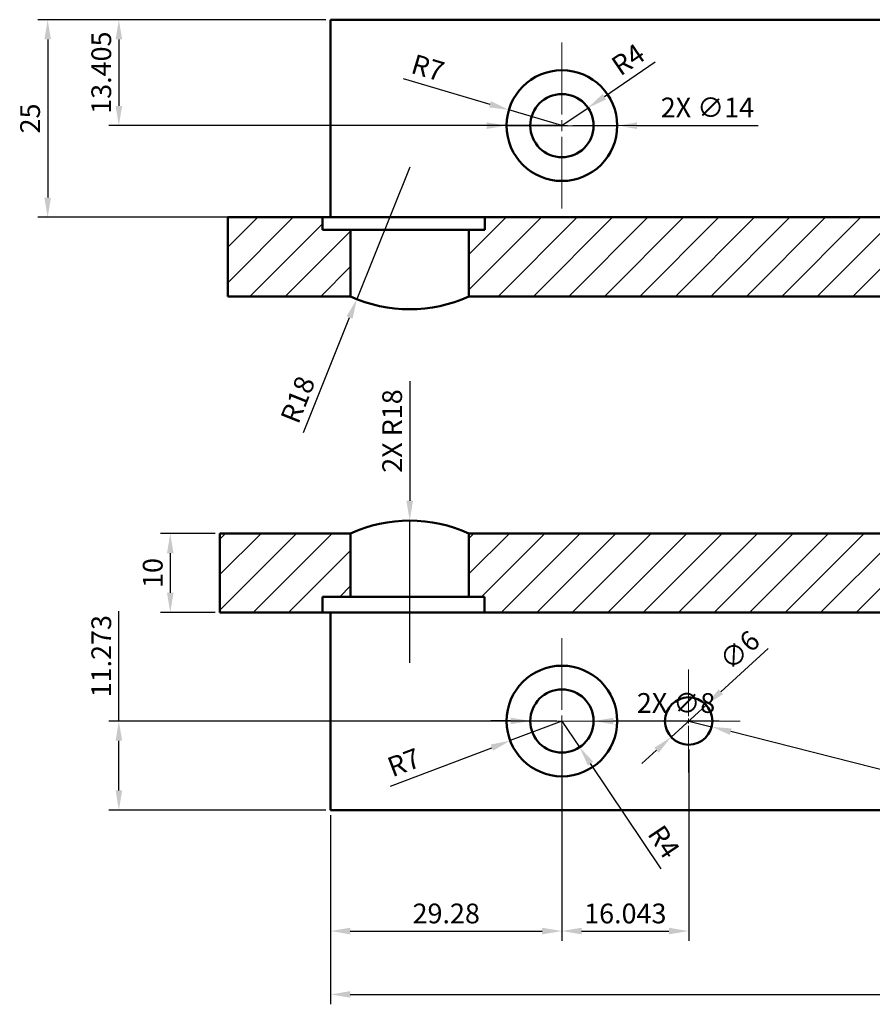
# Model space of a CAD drawing. Units: millimetres. Extents: x 1381 to 2009, y 1325 to 1613.
# Tile 1 of 6: x 1381 to 1489, y 1325 to 1450. Entities that reach past the tile are written whole.
import ezdxf

# ---------------------------------------------------------------- set-up
doc = ezdxf.new("R2010")
doc.units = ezdxf.units.MM
doc.linetypes.add('CENTER', pattern=[50.8, 31.75, -6.35, 6.35, -6.35])
for name, color, linetype, lineweight in [('M-CNTR', 1, 'CENTER', 18), ('M-DIMS', 2, 'Continuous', 25), ('M-HATC', 8, 'Continuous', 18), ('M-OUTL', 7, 'Continuous', 50)]:
    doc.layers.add(name, color=color, linetype=linetype, lineweight=lineweight)
doc.styles.get("Standard").update_dxf_attribs({"font": 'arial.ttf'})
doc.dimstyles.new('ISO-25', dxfattribs={"dimtxt": 2.5, "dimasz": 2.5, "dimexe": 1.25, "dimexo": 0.625, "dimtad": 1, "dimtxsty": 'Standard', "dimcen": 2.5, "dimadec": 0, "dimazin": 0, "dimtfac": 1, "dimtmove": 0, "dimatfit": 3, "dimfxl": 1, "dimarcsym": 0})

# ---------------------------------------------------------------- blocks, each defined once
blk = doc.blocks.new('*U3')
at = {"layer": 'M-CNTR', "color": 0, "transparency": 16777216}
for p, q in [((0, 1.4), (0, 10.5)), ((-10.5, 0), (-1.4, 0)), ((1.4, 0), (10.5, 0)), ((0, -10.5), (0, -1.4))]:
    blk.add_line(p, q, dxfattribs=at)
at = {"layer": 'M-CNTR', "color": 0, "linetype": 'Continuous', "transparency": 16777216}
for p, q in [((-0.7, 0), (0.7, 0)), ((0, -0.7), (0, 0.7))]:
    blk.add_line(p, q, dxfattribs=at)
blk = doc.blocks.new('*U4')
at = {"layer": 'M-CNTR', "color": 0, "transparency": 16777216}
for p, q in [((0, 1.4), (0, 10.5)), ((-10.5, 0), (-1.4, 0)), ((1.4, 0), (10.5, 0)), ((0, -10.5), (0, -1.4))]:
    blk.add_line(p, q, dxfattribs=at)
at = {"layer": 'M-CNTR', "color": 0, "linetype": 'Continuous', "transparency": 16777216}
for p, q in [((-0.7, 0), (0.7, 0)), ((0, -0.7), (0, 0.7))]:
    blk.add_line(p, q, dxfattribs=at)
blk = doc.blocks.new('*U5')
at = {"layer": 'M-CNTR', "color": 0, "transparency": 16777216}
for p, q in [((0, 0.6), (0, 6.5)), ((-6.5, 0), (-0.6, 0)), ((0.6, 0), (6.5, 0)), ((0, -6.5), (0, -0.6))]:
    blk.add_line(p, q, dxfattribs=at)
at = {"layer": 'M-CNTR', "color": 0, "linetype": 'Continuous', "transparency": 16777216}
for p, q in [((-0.3, 0), (0.3, 0)), ((0, -0.3), (0, 0.3))]:
    blk.add_line(p, q, dxfattribs=at)
blk = doc.blocks.new('*D38')
at = {"layer": 'Defpoints', "color": 0, "transparency": 16777216}
for p in [(1420.47, 1349.73), (1600.47, 1349.73), (1600.47, 1326.41)]:
    blk.add_point(p, dxfattribs=at)
at = {"layer": 'M-DIMS', "color": 0, "lineweight": -2, "transparency": 16777216}
for p, q in [((1420.47, 1349.11), (1420.47, 1325.16)), ((1600.47, 1349.11), (1600.47, 1325.16)), ((1422.97, 1326.41), (1597.97, 1326.41))]:
    blk.add_line(p, q, dxfattribs=at)
at = {"layer": 'M-DIMS', "color": 0, "transparency": 16777216}
for points in [[(1422.97, 1326.83), (1422.97, 1326), (1420.47, 1326.41)], [(1597.97, 1326.83), (1597.97, 1326), (1600.47, 1326.41)]]:
    blk.add_solid(points, dxfattribs=at)
at = {"layer": 'M-DIMS', "color": 0, "transparency": 16777216, "insert": (1510.47, 1328.31), "char_height": 2.5, "attachment_point": 5}
blk.add_mtext('180', dxfattribs=at)
blk = doc.blocks.new('*D40')
at = {"layer": 'Defpoints', "color": 0, "transparency": 16777216}
for p in [(1406.47, 1384.73), (1400.18, 1374.73), (1406.47, 1374.73)]:
    blk.add_point(p, dxfattribs=at)
at = {"layer": 'M-DIMS', "color": 0, "lineweight": -2, "transparency": 16777216}
for p, q in [((1405.85, 1384.73), (1398.93, 1384.73)), ((1400.18, 1382.23), (1400.18, 1377.23)), ((1405.85, 1374.73), (1398.93, 1374.73))]:
    blk.add_line(p, q, dxfattribs=at)
at = {"layer": 'M-DIMS', "color": 0, "transparency": 16777216}
for points in [[(1399.76, 1382.23), (1400.59, 1382.23), (1400.18, 1384.73)], [(1399.76, 1377.23), (1400.59, 1377.23), (1400.18, 1374.73)]]:
    blk.add_solid(points, dxfattribs=at)
at = {"layer": 'M-DIMS', "color": 0, "transparency": 16777216, "insert": (1398.28, 1379.73), "char_height": 2.5, "attachment_point": 5, "rotation": 90}
blk.add_mtext('10', dxfattribs=at)
blk = doc.blocks.new('*D52')
at = {"layer": 'Defpoints', "color": 0, "transparency": 16777216}
for p in [(1449.75, 1361), (1443.21, 1358.52)]:
    blk.add_point(p, dxfattribs=at)
at = {"layer": 'M-DIMS', "color": 0, "lineweight": -2, "transparency": 16777216}
for p, q in [((1449.75, 1361), (1443.21, 1358.52)), ((1428.06, 1352.77), (1440.87, 1357.63))]:
    blk.add_line(p, q, dxfattribs=at)
at = {"layer": 'M-DIMS', "color": 0, "transparency": 16777216}
blk.add_solid([(1440.73, 1358.02), (1441.02, 1357.24), (1443.21, 1358.52)], dxfattribs=at)
at = {"layer": 'M-DIMS', "color": 0, "transparency": 16777216, "insert": (1429.86, 1355.46), "char_height": 2.5, "attachment_point": 5, "rotation": 20.7916}
blk.add_mtext('R7', dxfattribs=at)
blk = doc.blocks.new('*D53')
at = {"layer": 'Defpoints', "color": 0, "transparency": 16777216}
for p in [(1449.75, 1361), (1451.99, 1357.68)]:
    blk.add_point(p, dxfattribs=at)
at = {"layer": 'M-DIMS', "color": 0, "lineweight": -2, "transparency": 16777216}
for p, q in [((1449.75, 1361), (1451.99, 1357.68)), ((1462.32, 1342.31), (1453.38, 1355.61))]:
    blk.add_line(p, q, dxfattribs=at)
at = {"layer": 'M-DIMS', "color": 0, "transparency": 16777216}
blk.add_solid([(1453.73, 1355.84), (1453.04, 1355.38), (1451.99, 1357.68)], dxfattribs=at)
at = {"layer": 'M-DIMS', "color": 0, "transparency": 16777216, "insert": (1462.4, 1345.55), "char_height": 2.5, "attachment_point": 5, "rotation": 303.9105}
blk.add_mtext('R4', dxfattribs=at)
blk = doc.blocks.new('*D54')
at = {"layer": 'Defpoints', "color": 0, "transparency": 16777216}
for p in [(1465.8, 1361), (1468.71, 1360.27)]:
    blk.add_point(p, dxfattribs=at)
at = {"layer": 'M-DIMS', "color": 0, "lineweight": -2, "transparency": 16777216}
for p, q in [((1465.8, 1361), (1468.71, 1360.27)), ((1513.03, 1349.08), (1471.13, 1359.66))]:
    blk.add_line(p, q, dxfattribs=at)
at = {"layer": 'M-DIMS', "color": 0, "transparency": 16777216}
blk.add_solid([(1471.23, 1360.06), (1471.03, 1359.25), (1468.71, 1360.27)], dxfattribs=at)
at = {"layer": 'M-DIMS', "color": 0, "transparency": 16777216, "insert": (1510.94, 1351.57), "char_height": 2.5, "attachment_point": 5, "rotation": 345.8378}
blk.add_mtext('R3', dxfattribs=at)
blk = doc.blocks.new('*D55')
at = {"layer": 'Defpoints', "color": 0, "transparency": 16777216}
for p in [(1443.04, 1438.32), (1449.75, 1436.33)]:
    blk.add_point(p, dxfattribs=at)
at = {"layer": 'M-DIMS', "color": 0, "lineweight": -2, "transparency": 16777216}
for p, q in [((1429.64, 1442.29), (1440.65, 1439.03)), ((1449.75, 1436.33), (1443.04, 1438.32))]:
    blk.add_line(p, q, dxfattribs=at)
at = {"layer": 'M-DIMS', "color": 0, "transparency": 16777216}
blk.add_solid([(1440.77, 1439.43), (1440.53, 1438.63), (1443.04, 1438.32)], dxfattribs=at)
at = {"layer": 'M-DIMS', "color": 0, "transparency": 16777216, "insert": (1432.7, 1443.34), "char_height": 2.5, "attachment_point": 5, "rotation": 343.4791}
blk.add_mtext('R7', dxfattribs=at)
blk = doc.blocks.new('*D56')
at = {"layer": 'Defpoints', "color": 0, "transparency": 16777216}
for p in [(1453.06, 1438.58), (1449.75, 1436.33)]:
    blk.add_point(p, dxfattribs=at)
at = {"layer": 'M-DIMS', "color": 0, "lineweight": -2, "transparency": 16777216}
for p, q in [((1461.55, 1444.36), (1455.13, 1439.99)), ((1449.75, 1436.33), (1453.06, 1438.58))]:
    blk.add_line(p, q, dxfattribs=at)
at = {"layer": 'M-DIMS', "color": 0, "transparency": 16777216}
blk.add_solid([(1454.89, 1440.33), (1455.36, 1439.64), (1453.06, 1438.58)], dxfattribs=at)
at = {"layer": 'M-DIMS', "color": 0, "transparency": 16777216, "insert": (1458.31, 1444.43), "char_height": 2.5, "attachment_point": 5, "rotation": 34.2814}
blk.add_mtext('R4', dxfattribs=at)
blk = doc.blocks.new('*D57')
at = {"layer": 'Defpoints', "color": 0, "transparency": 16777216}
for p in [(1420.47, 1449.73), (1384.66, 1424.73), (1419.43, 1424.73)]:
    blk.add_point(p, dxfattribs=at)
at = {"layer": 'M-DIMS', "color": 0, "lineweight": -2, "transparency": 16777216}
for p, q in [((1419.85, 1449.73), (1383.41, 1449.73)), ((1384.66, 1447.23), (1384.66, 1427.23)), ((1418.81, 1424.73), (1383.41, 1424.73))]:
    blk.add_line(p, q, dxfattribs=at)
at = {"layer": 'M-DIMS', "color": 0, "transparency": 16777216}
for points in [[(1384.24, 1447.23), (1385.08, 1447.23), (1384.66, 1449.73)], [(1384.24, 1427.23), (1385.08, 1427.23), (1384.66, 1424.73)]]:
    blk.add_solid(points, dxfattribs=at)
at = {"layer": 'M-DIMS', "color": 0, "transparency": 16777216, "insert": (1382.76, 1437.23), "char_height": 2.5, "attachment_point": 5, "rotation": 90}
blk.add_mtext('25', dxfattribs=at)
blk = doc.blocks.new('*D58')
at = {"layer": 'Defpoints', "color": 0, "transparency": 16777216}
for p in [(1430.49, 1431.09), (1423.8, 1414.38)]:
    blk.add_point(p, dxfattribs=at)
at = {"layer": 'M-DIMS', "color": 0, "lineweight": -2, "transparency": 16777216}
for p, q in [((1430.49, 1431.09), (1423.8, 1414.38)), ((1417.04, 1397.49), (1422.88, 1412.06))]:
    blk.add_line(p, q, dxfattribs=at)
at = {"layer": 'M-DIMS', "color": 0, "transparency": 16777216}
blk.add_solid([(1422.49, 1412.22), (1423.26, 1411.91), (1423.8, 1414.38)], dxfattribs=at)
at = {"layer": 'M-DIMS', "color": 0, "transparency": 16777216, "insert": (1416.62, 1401.55), "char_height": 2.5, "attachment_point": 5, "rotation": 68.1915}
blk.add_mtext('R18', dxfattribs=at)
blk = doc.blocks.new('*D93')
at = {"layer": 'Defpoints', "color": 0, "transparency": 16777216}
for p in [(1449.75, 1361), (1420.47, 1349.73), (1449.75, 1334.43)]:
    blk.add_point(p, dxfattribs=at)
at = {"layer": 'M-DIMS', "color": 0, "lineweight": -2, "transparency": 16777216}
for p, q in [((1449.75, 1360.38), (1449.75, 1333.18)), ((1420.47, 1349.11), (1420.47, 1333.18)), ((1422.97, 1334.43), (1447.25, 1334.43))]:
    blk.add_line(p, q, dxfattribs=at)
at = {"layer": 'M-DIMS', "color": 0, "transparency": 16777216}
for points in [[(1422.97, 1334.85), (1422.97, 1334.01), (1420.47, 1334.43)], [(1447.25, 1334.85), (1447.25, 1334.01), (1449.75, 1334.43)]]:
    blk.add_solid(points, dxfattribs=at)
at = {"layer": 'M-DIMS', "color": 0, "transparency": 16777216, "insert": (1435.11, 1336.33), "char_height": 2.5, "attachment_point": 5}
blk.add_mtext('29.28', dxfattribs=at)
blk = doc.blocks.new('*D94')
at = {"layer": 'Defpoints', "color": 0, "transparency": 16777216}
for p in [(1393.67, 1361), (1449.75, 1361), (1420.47, 1349.73)]:
    blk.add_point(p, dxfattribs=at)
at = {"layer": 'M-DIMS', "color": 0, "lineweight": -2, "transparency": 16777216}
for p, q in [((1393.67, 1361), (1393.67, 1374.9)), ((1449.13, 1361), (1392.42, 1361)), ((1393.67, 1352.23), (1393.67, 1358.5)), ((1419.85, 1349.73), (1392.42, 1349.73))]:
    blk.add_line(p, q, dxfattribs=at)
at = {"layer": 'M-DIMS', "color": 0, "transparency": 16777216}
for points in [[(1393.26, 1358.5), (1394.09, 1358.5), (1393.67, 1361)], [(1393.26, 1352.23), (1394.09, 1352.23), (1393.67, 1349.73)]]:
    blk.add_solid(points, dxfattribs=at)
at = {"layer": 'M-DIMS', "color": 0, "transparency": 16777216, "insert": (1391.77, 1369.2), "char_height": 2.5, "attachment_point": 5, "rotation": 90}
blk.add_mtext('11.273', dxfattribs=at)
blk = doc.blocks.new('*D95')
at = {"layer": 'Defpoints', "color": 0, "transparency": 16777216}
for p in [(1420.47, 1449.73), (1393.67, 1436.33), (1449.75, 1436.33)]:
    blk.add_point(p, dxfattribs=at)
at = {"layer": 'M-DIMS', "color": 0, "lineweight": -2, "transparency": 16777216}
for p, q in [((1419.85, 1449.73), (1392.42, 1449.73)), ((1393.67, 1447.23), (1393.67, 1438.83)), ((1449.13, 1436.33), (1392.42, 1436.33))]:
    blk.add_line(p, q, dxfattribs=at)
at = {"layer": 'M-DIMS', "color": 0, "transparency": 16777216}
for points in [[(1393.26, 1447.23), (1394.09, 1447.23), (1393.67, 1449.73)], [(1393.26, 1438.83), (1394.09, 1438.83), (1393.67, 1436.33)]]:
    blk.add_solid(points, dxfattribs=at)
at = {"layer": 'M-DIMS', "color": 0, "transparency": 16777216, "insert": (1391.77, 1443.03), "char_height": 2.5, "attachment_point": 5, "rotation": 90}
blk.add_mtext('13.405', dxfattribs=at)
blk = doc.blocks.new('*D96')
at = {"layer": 'Defpoints', "color": 0, "transparency": 16777216}
for p in [(1449.75, 1361), (1465.8, 1358), (1465.8, 1334.43)]:
    blk.add_point(p, dxfattribs=at)
at = {"layer": 'M-DIMS', "color": 0, "lineweight": -2, "transparency": 16777216}
for p, q in [((1449.75, 1360.38), (1449.75, 1333.18)), ((1465.8, 1357.38), (1465.8, 1333.18)), ((1452.25, 1334.43), (1463.3, 1334.43))]:
    blk.add_line(p, q, dxfattribs=at)
at = {"layer": 'M-DIMS', "color": 0, "transparency": 16777216}
for points in [[(1452.25, 1334.85), (1452.25, 1334.01), (1449.75, 1334.43)], [(1463.3, 1334.85), (1463.3, 1334.01), (1465.8, 1334.43)]]:
    blk.add_solid(points, dxfattribs=at)
at = {"layer": 'M-DIMS', "color": 0, "transparency": 16777216, "insert": (1457.78, 1336.33), "char_height": 2.5, "attachment_point": 5}
blk.add_mtext('16.043', dxfattribs=at)
blk = doc.blocks.new('*D122')
at = {"layer": 'Defpoints', "color": 0, "transparency": 16777216}
for p in [(1442.75, 1436.33), (1456.75, 1436.32)]:
    blk.add_point(p, dxfattribs=at)
at = {"layer": 'M-DIMS', "color": 0, "lineweight": -2, "transparency": 16777216}
for p, q in [((1440.25, 1436.33), (1437.75, 1436.33)), ((1442.75, 1436.33), (1456.75, 1436.32)), ((1474.58, 1436.32), (1459.25, 1436.32))]:
    blk.add_line(p, q, dxfattribs=at)
at = {"layer": 'M-DIMS', "color": 0, "transparency": 16777216}
for points in [[(1440.25, 1436.74), (1440.25, 1435.91), (1442.75, 1436.33)], [(1459.25, 1436.74), (1459.25, 1435.91), (1456.75, 1436.32)]]:
    blk.add_solid(points, dxfattribs=at)
at = {"layer": 'M-DIMS', "color": 0, "transparency": 16777216, "insert": (1468.17, 1438.3), "char_height": 2.5, "attachment_point": 5, "rotation": 359.9988}
blk.add_mtext('2X ∅14', dxfattribs=at)
blk = doc.blocks.new('*D123')
at = {"layer": 'Defpoints', "color": 0, "transparency": 16777216}
for p in [(1445.75, 1361.01), (1453.75, 1361)]:
    blk.add_point(p, dxfattribs=at)
at = {"layer": 'M-DIMS', "color": 0, "lineweight": -2, "transparency": 16777216}
for p, q in [((1443.25, 1361.01), (1440.75, 1361.01)), ((1445.75, 1361.01), (1453.75, 1361)), ((1469.65, 1360.99), (1456.25, 1361))]:
    blk.add_line(p, q, dxfattribs=at)
at = {"layer": 'M-DIMS', "color": 0, "transparency": 16777216}
for points in [[(1443.26, 1361.43), (1443.25, 1360.59), (1445.75, 1361.01)], [(1456.26, 1361.41), (1456.25, 1360.58), (1453.75, 1361)]]:
    blk.add_solid(points, dxfattribs=at)
at = {"layer": 'M-DIMS', "color": 0, "transparency": 16777216, "insert": (1464.2, 1362.96), "char_height": 2.5, "attachment_point": 5, "rotation": 359.9545}
blk.add_mtext('2X ∅8', dxfattribs=at)
blk = doc.blocks.new('*D124')
at = {"layer": 'Defpoints', "color": 0, "transparency": 16777216}
for p in [(1468.02, 1363.02), (1463.58, 1358.98)]:
    blk.add_point(p, dxfattribs=at)
at = {"layer": 'M-DIMS', "color": 0, "lineweight": -2, "transparency": 16777216}
for p, q in [((1475.86, 1370.17), (1469.86, 1364.71)), ((1463.58, 1358.98), (1468.02, 1363.02)), ((1461.73, 1357.3), (1459.88, 1355.62))]:
    blk.add_line(p, q, dxfattribs=at)
at = {"layer": 'M-DIMS', "color": 0, "transparency": 16777216}
for points in [[(1469.58, 1365.01), (1470.14, 1364.4), (1468.02, 1363.02)], [(1461.45, 1357.61), (1462.01, 1356.99), (1463.58, 1358.98)]]:
    blk.add_solid(points, dxfattribs=at)
at = {"layer": 'M-DIMS', "color": 0, "transparency": 16777216, "insert": (1472.46, 1369.73), "char_height": 2.5, "attachment_point": 5, "rotation": 42.3234}
blk.add_mtext('∅6', dxfattribs=at)
blk = doc.blocks.new('*D125')
at = {"layer": 'Defpoints', "color": 0, "transparency": 16777216}
for p in [(1430.49, 1386.37), (1430.49, 1368.37)]:
    blk.add_point(p, dxfattribs=at)
at = {"layer": 'M-DIMS', "color": 0, "lineweight": -2, "transparency": 16777216}
for p, q in [((1430.49, 1404.01), (1430.49, 1388.87)), ((1430.49, 1368.37), (1430.49, 1386.37))]:
    blk.add_line(p, q, dxfattribs=at)
at = {"layer": 'M-DIMS', "color": 0, "transparency": 16777216}
blk.add_solid([(1430.07, 1388.87), (1430.91, 1388.87), (1430.49, 1386.37)], dxfattribs=at)
at = {"layer": 'M-DIMS', "color": 0, "transparency": 16777216, "insert": (1428.59, 1397.69), "char_height": 2.5, "attachment_point": 5, "rotation": 89.9997}
blk.add_mtext('2X R18', dxfattribs=at)

msp = doc.modelspace()

# ---------------------------------------------------------------- hatches: boundary and pattern name
at = {"layer": 'M-HATC'}
h = msp.add_hatch(dxfattribs=at)
h.set_pattern_fill('ANSI31', color=256)
h.paths.add_polyline_path([(1422.9909, 1423.1434), (1419.4301, 1423.1434), (1419.4301, 1424.7301), (1407.4722, 1424.7301), (1407.4722, 1414.7301), (1422.9909, 1414.7301)])
h.paths.add_polyline_path([(1506.2792, 1420.796), (1506.2792, 1429.7301), (1532.6154, 1429.7301, -0.40409142), (1534.5583, 1431.7171), (1534.4722, 1434.7301), (1497.4722, 1434.7301), (1497.4722, 1424.7301), (1439.9762, 1424.7301), (1439.9762, 1423.1434), (1437.9909, 1423.1434), (1437.9909, 1414.7301), (1502.746, 1414.7301, -0.04886567)])
h.paths.add_polyline_path([(1507.1646, 1384.7301), (1437.9909, 1384.7301), (1437.9909, 1376.7301), (1439.9421, 1376.7301), (1439.9401, 1374.7301), (1501.4722, 1374.7301), (1501.4722, 1364.7301), (1536.4722, 1364.7301), (1536.3861, 1367.7432, -0.42260463), (1534.329, 1369.7424, -0.40587199), (1536.2718, 1371.7415), (1536.2216, 1373.5004), (1507.1646, 1373.5004)])
h.paths.add_polyline_path([(1422.9909, 1384.7301), (1406.4722, 1384.7301), (1406.4722, 1374.7301), (1419.4301, 1374.7301), (1419.4301, 1376.7301), (1422.9909, 1376.7301)])
h.paths.add_polyline_path([(1571.4722, 1399.7301, -0.18599034), (1562.1646, 1375.5741), (1562.1646, 1373.5004), (1550.0325, 1373.5004, -0.10324325), (1538.3251, 1369.8661, -0.42401254), (1536.3861, 1367.7432), (1536.4722, 1364.7301), (1571.4722, 1364.7301)])

# ---------------------------------------------------------------- linework, layer by layer
at = {"layer": 'M-OUTL'}
for p, q in [((1420.4722, 1449.7301), (1600.4722, 1449.7301)), ((1420.4722, 1424.7301), (1420.4722, 1449.7301)), ((1497.4722, 1424.7301), (1407.4722, 1424.7301)), ((1407.4722, 1424.7301), (1407.4722, 1414.7301)), ((1419.4301, 1424.7301), (1419.4301, 1423.1434)), ((1439.9762, 1423.1434), (1439.9762, 1424.7301)), ((1419.4301, 1423.1434), (1439.9762, 1423.1434)), ((1422.9909, 1423.1434), (1422.9909, 1414.7301)), ((1437.9909, 1414.7301), (1437.9909, 1423.1434)), ((1407.4722, 1414.7301), (1422.9909, 1414.7301)), ((1437.9909, 1414.7301), (1506.2792, 1414.7301)), ((1406.4722, 1374.7301), (1406.4722, 1384.7301)), ((1406.4722, 1384.7301), (1422.9909, 1384.7301)), ((1422.9909, 1384.7301), (1422.9909, 1376.7301)), ((1437.9909, 1376.7301), (1437.9909, 1384.7301)), ((1437.9909, 1384.7301), (1507.1646, 1384.7301)), ((1419.4301, 1374.7301), (1419.4301, 1376.7301)), ((1419.4301, 1376.7301), (1439.9421, 1376.7301)), ((1439.9421, 1376.7301), (1439.9401, 1374.7301)), ((1501.4722, 1374.7301), (1406.4722, 1374.7301)), ((1420.4722, 1349.7301), (1420.4722, 1374.7301)), ((1600.4722, 1349.7301), (1420.4722, 1349.7301))]:
    msp.add_line(p, q, dxfattribs=at)
for centre, radius in [((1449.7547, 1436.3252), 7), ((1449.7547, 1436.3252), 4), ((1449.7547, 1361.0032), 7), ((1449.7547, 1361.0032), 4), ((1465.7975, 1361.0032), 3)]:
    msp.add_circle(centre, radius, dxfattribs=at)
for centre, start, end in [((1430.4909, 1431.0932), 245.375682, 294.624318), ((1430.4909, 1368.3671), 65.375682, 114.624318)]:
    msp.add_arc(centre, 18, start, end, dxfattribs=at)

# ---------------------------------------------------------------- block references
at = {"layer": 'M-CNTR'}
for name, p in [('*U3', (1449.7547, 1436.3252)), ('*U4', (1449.7547, 1361.0032)), ('*U5', (1465.7975, 1361.0032))]:
    msp.add_blockref(name, p, dxfattribs=at)

# ---------------------------------------------------------------- dimensions: what is measured, and where the dimension line sits
at = {"layer": 'M-DIMS'}
for base, p1, p2, override, picture, middle in [((1384.6588, 1424.7301), (1420.4722, 1449.7301), (1419.4301, 1424.7301), {"dimclrd": 0, "dimclre": 0, "dimclrt": 0}, '*D57', (1382.7574, 1437.2301)), ((1393.6722, 1436.3252), (1420.4722, 1449.7301), (1449.7547, 1436.3252), {"dimdec": 3, "dimlfac": 1, "dimrnd": 0, "dimzin": 0, "dimdsep": 46, "dimlunit": 2}, '*D95', (1391.7699, 1443.0276)), ((1400.1782, 1374.7301), (1406.4722, 1384.7301), (1406.4722, 1374.7301), {"dimclrd": 0, "dimclre": 0, "dimclrt": 0}, '*D40', (1398.2767, 1379.7301)), ((1393.6722, 1361.0032), (1420.4722, 1349.7301), (1449.7547, 1361.0032), {"dimdec": 3, "dimlfac": 1, "dimrnd": 0, "dimzin": 0, "dimdsep": 46, "dimlunit": 2}, '*D94', (1391.7699, 1369.1998))]:
    dim = msp.add_linear_dim(base=base, p1=p1, p2=p2, angle=90, dimstyle='ISO-25', override=override, dxfattribs=at)
    dim.commit()
    dim.dimension.update_dxf_attribs({"geometry": picture, "text_midpoint": middle})
dim = msp.add_radius_dim(center=(1449.7547, 1436.3252), mpoint=(1453.0598, 1438.5782), dimstyle='ISO-25', override={"dimclrd": 0, "dimclre": 0, "dimclrt": 0}, dxfattribs=at)
dim.commit()
dim.dimension.update_dxf_attribs({"geometry": '*D56', "text_midpoint": (1458.3128, 1444.4283)})
for center, mpoint, picture, middle in [((1449.7547, 1436.3252), (1443.0437, 1438.3157), '*D55', (1432.1703, 1441.5409)), ((1430.4909, 1431.0932), (1423.8038, 1414.3814), '*D58', (1418.387, 1400.8443)), ((1449.7547, 1361.0032), (1443.2105, 1358.5184), '*D52', (1430.5288, 1353.7031)), ((1449.7547, 1361.0032), (1451.9863, 1357.6835), '*D53', (1460.8487, 1344.5001)), ((1465.7975, 1361.0032), (1468.7063, 1360.2692), '*D54', (1510.4722, 1349.7301))]:
    dim = msp.add_radius_dim(center=center, mpoint=mpoint, dimstyle='ISO-25', override={"dimclrd": 0, "dimclre": 0, "dimclrt": 0}, dxfattribs=at)
    dim.commit()
    dim.dimension.update_dxf_attribs({"geometry": picture, "text_midpoint": middle, "dimtype": 164})
dim = msp.add_diameter_dim_2p(p1=(1442.7547, 1436.3253), p2=(1456.7547, 1436.325), text='2X <>', dimstyle='ISO-25', override={"dimdec": 0, "dimlfac": 1, "dimrnd": 0, "dimzin": 0, "dimdsep": 46, "dimlunit": 2}, dxfattribs=at)
dim.commit()
dim.dimension.update_dxf_attribs({"geometry": '*D122', "text_midpoint": (1468.1658, 1436.3248)})
dim = msp.add_radius_dim(center=(1430.4909, 1368.3671), mpoint=(1430.491, 1386.3671), text='2X <>', dimstyle='ISO-25', override={"dimdec": 0, "dimlfac": 1, "dimrnd": 0, "dimzin": 0, "dimdsep": 46, "dimlunit": 2}, dxfattribs=at)
dim.commit()
dim.dimension.update_dxf_attribs({"geometry": '*D125', "text_midpoint": (1428.5896, 1397.6887)})
dim = msp.add_diameter_dim_2p(p1=(1463.5794, 1358.9832), p2=(1468.0156, 1363.0231), dimstyle='ISO-25', override={"dimdec": 0, "dimlfac": 1, "dimrnd": 0, "dimzin": 0, "dimdsep": 46, "dimlunit": 2}, dxfattribs=at)
dim.commit()
dim.dimension.update_dxf_attribs({"geometry": '*D124', "text_midpoint": (1473.7852, 1368.2774)})
dim = msp.add_diameter_dim_2p(p1=(1445.7547, 1361.0064), p2=(1453.7547, 1361), text='2X <>', dimstyle='ISO-25', override={"dimdec": 0, "dimlfac": 1, "dimrnd": 0, "dimzin": 0, "dimdsep": 46, "dimlunit": 2}, dxfattribs=at)
dim.commit()
dim.dimension.update_dxf_attribs({"geometry": '*D123', "text_midpoint": (1464.2023, 1360.9917), "dimtype": 163})
for base, p1, p2, override, picture, middle in [((1449.7547, 1334.4301), (1420.4722, 1349.7301), (1449.7547, 1361.0032), {"dimdec": 2, "dimlfac": 1, "dimrnd": 0, "dimzin": 0, "dimdsep": 46, "dimlunit": 2}, '*D93', (1435.1134, 1336.3316)), ((1465.7975, 1334.4301), (1449.7547, 1361.0032), (1465.7975, 1358.0032), {"dimdec": 3, "dimlfac": 1, "dimrnd": 0, "dimzin": 0, "dimdsep": 46, "dimlunit": 2}, '*D96', (1457.7761, 1336.3324)), ((1600.4722, 1326.4121), (1420.4722, 1349.7301), (1600.4722, 1349.7301), {"dimclrd": 0, "dimclre": 0, "dimclrt": 0}, '*D38', (1510.4722, 1328.3136))]:
    dim = msp.add_linear_dim(base=base, p1=p1, p2=p2, dimstyle='ISO-25', override=override, dxfattribs=at)
    dim.commit()
    dim.dimension.update_dxf_attribs({"geometry": picture, "text_midpoint": middle})

doc.saveas('drawing.dxf')
